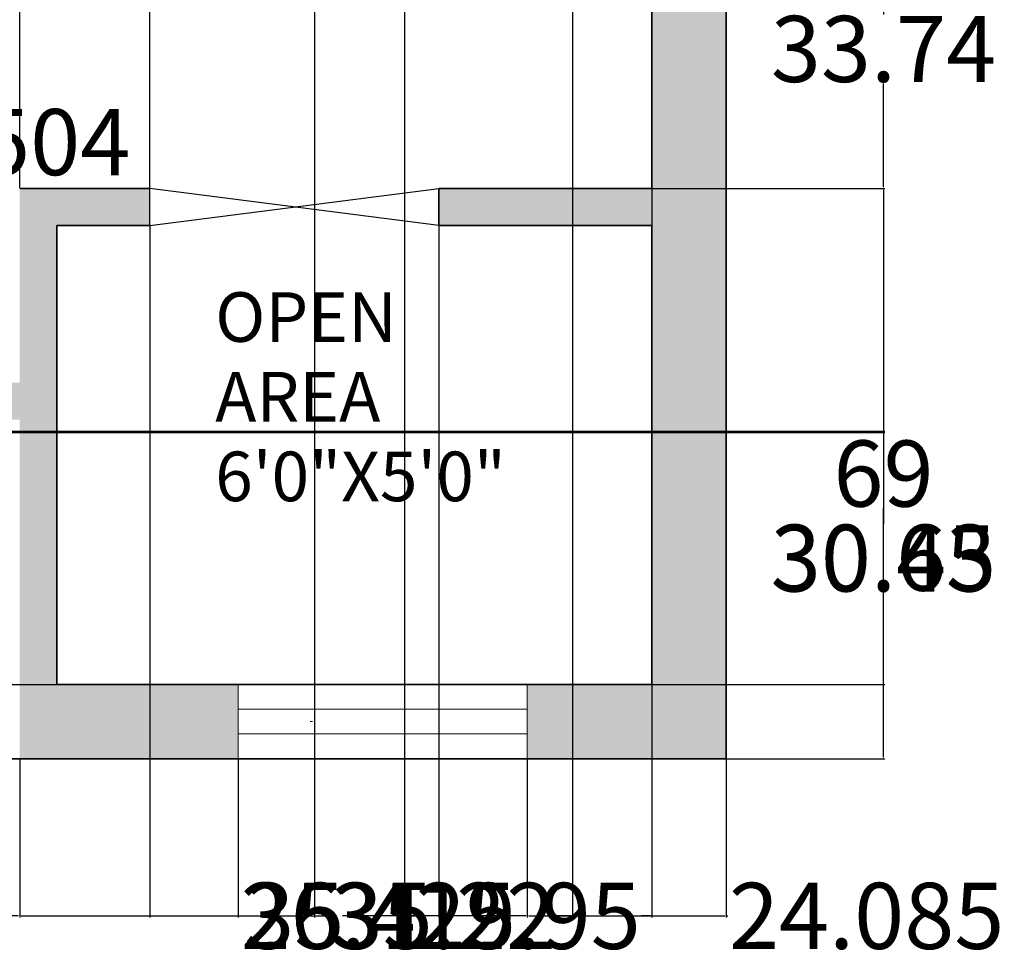
# Model space of a CAD drawing. Units: inches. Extents: x -24 to 368, y -370 to 58.
# Tile 4 of 9: x 237 to 356, y -369 to -255. Entities that reach past the tile are written whole.
import ezdxf

# ---------------------------------------------------------------- set-up
doc = ezdxf.new("R2010")
doc.units = ezdxf.units.IN
doc.header["$MEASUREMENT"] = 0
for name, color, linetype, lineweight in [('A-ANNO-DIMS', 2, 'Continuous', 18), ('A-AREA-IDEN', 7, 'Continuous', 18), ('A-WALL', 7, 'Continuous', 35)]:
    doc.layers.add(name, color=color, linetype=linetype, lineweight=lineweight)
for name, color, linetype, lineweight, true_color in [('A-DOOR', 40, 'Continuous', 25, 0xf8d731), ('A-GLAZ', 30, 'Continuous', 18, 0xf26722), ('A-WALL-PATT', 18, 'Continuous', 13, 0x000000)]:
    doc.layers.add(name, color=color, linetype=linetype, lineweight=lineweight, true_color=true_color)
doc.styles.get("Standard").update_dxf_attribs({"font": 'arial.ttf'})
doc.dimstyles.get("Standard").update_dxf_attribs({"dimtxt": 8, "dimasz": 0.18, "dimexe": 0.18, "dimexo": 0.0625, "dimgap": 0.09, "dimtad": 0, "dimtih": 1, "dimtoh": 1, "dimdec": 4, "dimzin": 0, "dimdsep": 46, "dimlunit": 3, "dimtxsty": 'Standard', "dimcen": 0.09, "dimclre": 5, "dimclrt": 6, "dimadec": 0, "dimazin": 0, "dimtfac": 1, "dimtdec": 4, "dimtofl": 0, "dimtmove": 0, "dimatfit": 3, "dimfxl": 1, "dimtolj": 1, "dimtzin": 0, "dimarcsym": 0})

# ---------------------------------------------------------------- blocks, each defined once
blk = doc.blocks.new('*D29')
at = {"layer": 'A-ANNO-DIMS', "color": 5, "lineweight": -2, "transparency": 16777216}
for p, q in [((131.66, -344.42), (131.66, -363.55)), ((236.66, -344.42), (236.66, -363.55))]:
    blk.add_line(p, q, dxfattribs=at)
at = {"layer": 'A-ANNO-DIMS', "color": 0, "lineweight": -2, "transparency": 16777216}
for p, q in [((131.84, -363.37), (175.58, -363.37)), ((236.48, -363.37), (192.74, -363.37))]:
    blk.add_line(p, q, dxfattribs=at)
at = {"layer": 'A-ANNO-DIMS', "color": 0, "transparency": 16777216}
for points in [[(131.84, -363.34), (131.84, -363.4), (131.66, -363.37)], [(236.48, -363.34), (236.48, -363.4), (236.66, -363.37)]]:
    blk.add_solid(points, dxfattribs=at)
at = {"layer": 'Defpoints', "color": 0, "transparency": 16777216}
for p in [(131.66, -344.36), (236.66, -344.36), (236.66, -363.37)]:
    blk.add_point(p, dxfattribs=at)
at = {"layer": 'A-ANNO-DIMS', "color": 6, "transparency": 16777216, "insert": (184.16, -363.37), "char_height": 8, "attachment_point": 5}
blk.add_mtext('\\A1;105', dxfattribs=at)
blk = doc.blocks.new('*D30')
at = {"layer": 'A-ANNO-DIMS', "color": 5, "lineweight": -2, "transparency": 16777216}
for p, q in [((236.66, -344.42), (236.66, -363.55)), ((263.08, -344.42), (263.08, -363.55))]:
    blk.add_line(p, q, dxfattribs=at)
at = {"layer": 'A-ANNO-DIMS', "color": 0, "lineweight": -2, "transparency": 16777216}
for p, q in [((236.84, -363.37), (262.9, -363.37)), ((263.08, -363.37), (263.26, -363.37))]:
    blk.add_line(p, q, dxfattribs=at)
at = {"layer": 'A-ANNO-DIMS', "color": 0, "transparency": 16777216}
for points in [[(236.84, -363.34), (236.84, -363.4), (236.66, -363.37)], [(262.9, -363.34), (262.9, -363.4), (263.08, -363.37)]]:
    blk.add_solid(points, dxfattribs=at)
at = {"layer": 'Defpoints', "color": 0, "transparency": 16777216}
for p in [(236.66, -344.36), (263.08, -344.36), (263.08, -363.37)]:
    blk.add_point(p, dxfattribs=at)
at = {"layer": 'A-ANNO-DIMS', "color": 6, "transparency": 16777216, "insert": (280.05, -363.37), "char_height": 8, "attachment_point": 5}
blk.add_mtext('\\A1;26.415', dxfattribs=at)
blk = doc.blocks.new('*D31')
at = {"layer": 'A-ANNO-DIMS', "color": 5, "lineweight": -2, "transparency": 16777216}
for p, q in [((263.08, -344.42), (263.08, -363.55)), ((298.08, -344.42), (298.08, -363.55))]:
    blk.add_line(p, q, dxfattribs=at)
at = {"layer": 'A-ANNO-DIMS', "color": 0, "lineweight": -2, "transparency": 16777216}
for p, q in [((263.26, -363.37), (274.73, -363.37)), ((297.9, -363.37), (286.42, -363.37))]:
    blk.add_line(p, q, dxfattribs=at)
at = {"layer": 'A-ANNO-DIMS', "color": 0, "transparency": 16777216}
for points in [[(263.26, -363.34), (263.26, -363.4), (263.08, -363.37)], [(297.9, -363.34), (297.9, -363.4), (298.08, -363.37)]]:
    blk.add_solid(points, dxfattribs=at)
at = {"layer": 'Defpoints', "color": 0, "transparency": 16777216}
for p in [(263.08, -344.36), (298.08, -344.36), (298.08, -363.37)]:
    blk.add_point(p, dxfattribs=at)
at = {"layer": 'A-ANNO-DIMS', "color": 6, "transparency": 16777216, "insert": (280.58, -363.37), "char_height": 8, "attachment_point": 5}
blk.add_mtext('\\A1;35', dxfattribs=at)
blk = doc.blocks.new('*D32')
at = {"layer": 'A-ANNO-DIMS', "color": 5, "lineweight": -2, "transparency": 16777216}
for p, q in [((298.08, -344.42), (298.08, -363.55)), ((322.16, -344.42), (322.16, -363.55))]:
    blk.add_line(p, q, dxfattribs=at)
at = {"layer": 'A-ANNO-DIMS', "color": 0, "lineweight": -2, "transparency": 16777216}
for p, q in [((298.26, -363.37), (321.98, -363.37)), ((322.16, -363.37), (322.34, -363.37))]:
    blk.add_line(p, q, dxfattribs=at)
at = {"layer": 'A-ANNO-DIMS', "color": 0, "transparency": 16777216}
for points in [[(298.26, -363.34), (298.26, -363.4), (298.08, -363.37)], [(321.98, -363.34), (321.98, -363.4), (322.16, -363.37)]]:
    blk.add_solid(points, dxfattribs=at)
at = {"layer": 'Defpoints', "color": 0, "transparency": 16777216}
for p in [(298.08, -344.36), (322.16, -344.36), (322.16, -363.37)]:
    blk.add_point(p, dxfattribs=at)
at = {"layer": 'A-ANNO-DIMS', "color": 6, "transparency": 16777216, "insert": (339.14, -363.37), "char_height": 8, "attachment_point": 5}
blk.add_mtext('\\A1;24.085', dxfattribs=at)
blk = doc.blocks.new('*D33')
at = {"layer": 'A-ANNO-DIMS', "color": 5, "lineweight": -2, "transparency": 16777216}
for p, q in [((313.22, -275.36), (341.36, -275.36)), ((322.22, -344.36), (341.36, -344.36))]:
    blk.add_line(p, q, dxfattribs=at)
at = {"layer": 'A-ANNO-DIMS', "color": 0, "lineweight": -2, "transparency": 16777216}
for p, q in [((341.18, -275.54), (341.18, -305.68)), ((341.18, -344.18), (341.18, -314.03))]:
    blk.add_line(p, q, dxfattribs=at)
at = {"layer": 'A-ANNO-DIMS', "color": 0, "transparency": 16777216}
for points in [[(341.15, -275.54), (341.21, -275.54), (341.18, -275.36)], [(341.15, -344.18), (341.21, -344.18), (341.18, -344.36)]]:
    blk.add_solid(points, dxfattribs=at)
at = {"layer": 'Defpoints', "color": 0, "transparency": 16777216}
for p in [(313.16, -275.36), (341.18, -275.36), (322.16, -344.36)]:
    blk.add_point(p, dxfattribs=at)
at = {"layer": 'A-ANNO-DIMS', "color": 6, "transparency": 16777216, "insert": (341.18, -309.86), "char_height": 8, "attachment_point": 5}
blk.add_mtext('\\A1;69', dxfattribs=at)
blk = doc.blocks.new('*D34')
at = {"layer": 'A-ANNO-DIMS', "color": 5, "lineweight": -2, "transparency": 16777216}
for p, q in [((322.22, -241.61), (341.36, -241.61)), ((313.22, -275.36), (341.36, -275.36))]:
    blk.add_line(p, q, dxfattribs=at)
at = {"layer": 'A-ANNO-DIMS', "color": 0, "lineweight": -2, "transparency": 16777216}
for p, q in [((341.18, -241.79), (341.18, -254.31)), ((341.18, -275.18), (341.18, -262.66))]:
    blk.add_line(p, q, dxfattribs=at)
at = {"layer": 'A-ANNO-DIMS', "color": 0, "transparency": 16777216}
for points in [[(341.15, -241.79), (341.21, -241.79), (341.18, -241.61)], [(341.15, -275.18), (341.21, -275.18), (341.18, -275.36)]]:
    blk.add_solid(points, dxfattribs=at)
at = {"layer": 'Defpoints', "color": 0, "transparency": 16777216}
for p in [(322.16, -241.61), (341.18, -241.61), (313.16, -275.36)]:
    blk.add_point(p, dxfattribs=at)
at = {"layer": 'A-ANNO-DIMS', "color": 6, "transparency": 16777216, "insert": (341.18, -258.49), "char_height": 8, "attachment_point": 5}
blk.add_mtext('\\A1;33.74', dxfattribs=at)
blk = doc.blocks.new('*D43')
at = {"layer": 'A-ANNO-DIMS', "color": 5, "lineweight": -2, "transparency": 16777216}
for p, q in [((283.21, 24.58), (283.21, -363.55)), ((313.16, 24.58), (313.16, -363.55))]:
    blk.add_line(p, q, dxfattribs=at)
at = {"layer": 'A-ANNO-DIMS', "color": 0, "lineweight": -2, "transparency": 16777216}
for p, q in [((283.39, -363.37), (284.5, -363.37)), ((312.98, -363.37), (311.87, -363.37))]:
    blk.add_line(p, q, dxfattribs=at)
at = {"layer": 'A-ANNO-DIMS', "color": 0, "transparency": 16777216}
for points in [[(283.39, -363.34), (283.39, -363.4), (283.21, -363.37)], [(312.98, -363.34), (312.98, -363.4), (313.16, -363.37)]]:
    blk.add_solid(points, dxfattribs=at)
at = {"layer": 'Defpoints', "color": 0, "transparency": 16777216}
for p in [(283.21, 24.64), (313.16, 24.64), (313.16, -363.37)]:
    blk.add_point(p, dxfattribs=at)
at = {"layer": 'A-ANNO-DIMS', "color": 6, "transparency": 16777216, "insert": (298.19, -363.37), "char_height": 8, "attachment_point": 5}
blk.add_mtext('\\A1;29.95', dxfattribs=at)
blk = doc.blocks.new('*D46')
at = {"layer": 'A-ANNO-DIMS', "color": 5, "lineweight": -2, "transparency": 16777216}
for p, q in [((13.22, -304.91), (341.36, -304.91)), ((13.22, -335.36), (341.36, -335.36))]:
    blk.add_line(p, q, dxfattribs=at)
at = {"layer": 'A-ANNO-DIMS', "color": 0, "lineweight": -2, "transparency": 16777216}
for p, q in [((341.18, -305.09), (341.18, -315.95)), ((341.18, -335.18), (341.18, -324.31))]:
    blk.add_line(p, q, dxfattribs=at)
at = {"layer": 'A-ANNO-DIMS', "color": 0, "transparency": 16777216}
for points in [[(341.15, -305.09), (341.21, -305.09), (341.18, -304.91)], [(341.15, -335.18), (341.21, -335.18), (341.18, -335.36)]]:
    blk.add_solid(points, dxfattribs=at)
at = {"layer": 'Defpoints', "color": 0, "transparency": 16777216}
for p in [(13.16, -304.91), (341.18, -304.91), (13.16, -335.36)]:
    blk.add_point(p, dxfattribs=at)
at = {"layer": 'A-ANNO-DIMS', "color": 6, "transparency": 16777216, "insert": (341.18, -320.13), "char_height": 8, "attachment_point": 5}
blk.add_mtext('\\A1;30.45', dxfattribs=at)
blk = doc.blocks.new('*D61')
at = {"layer": 'A-ANNO-DIMS', "color": 5, "lineweight": -2, "transparency": 16777216}
for p, q in [((236.66, -275.29), (236.66, 52.85)), ((252.39, -275.29), (252.39, 52.85))]:
    blk.add_line(p, q, dxfattribs=at)
at = {"layer": 'A-ANNO-DIMS', "color": 0, "lineweight": -2, "transparency": 16777216}
for p, q in [((236.84, 52.67), (252.21, 52.67)), ((252.39, 52.67), (252.57, 52.67))]:
    blk.add_line(p, q, dxfattribs=at)
at = {"layer": 'A-ANNO-DIMS', "color": 0, "transparency": 16777216}
for points in [[(236.84, 52.7), (236.84, 52.64), (236.66, 52.67)], [(252.21, 52.7), (252.21, 52.64), (252.39, 52.67)]]:
    blk.add_solid(points, dxfattribs=at)
at = {"layer": 'Defpoints', "color": 0, "transparency": 16777216}
for p in [(252.39, 52.67), (236.66, -275.36), (252.39, -275.36)]:
    blk.add_point(p, dxfattribs=at)
at = {"layer": 'A-ANNO-DIMS', "color": 6, "transparency": 16777216, "insert": (265.78, 52.67), "char_height": 8, "attachment_point": 5}
blk.add_mtext('\\A1;15.73', dxfattribs=at)
blk = doc.blocks.new('*D62')
at = {"layer": 'A-ANNO-DIMS', "color": 5, "lineweight": -2, "transparency": 16777216}
for p, q in [((252.39, -279.92), (252.39, -363.55)), ((287.39, -279.92), (287.39, -363.55))]:
    blk.add_line(p, q, dxfattribs=at)
at = {"layer": 'A-ANNO-DIMS', "color": 0, "lineweight": -2, "transparency": 16777216}
for p, q in [((252.57, -363.37), (264.04, -363.37)), ((287.21, -363.37), (275.74, -363.37))]:
    blk.add_line(p, q, dxfattribs=at)
at = {"layer": 'A-ANNO-DIMS', "color": 0, "transparency": 16777216}
for points in [[(252.57, -363.34), (252.57, -363.4), (252.39, -363.37)], [(287.21, -363.34), (287.21, -363.4), (287.39, -363.37)]]:
    blk.add_solid(points, dxfattribs=at)
at = {"layer": 'Defpoints', "color": 0, "transparency": 16777216}
for p in [(252.39, -279.86), (287.39, -279.86), (287.39, -363.37)]:
    blk.add_point(p, dxfattribs=at)
at = {"layer": 'A-ANNO-DIMS', "color": 6, "transparency": 16777216, "insert": (269.89, -363.37), "char_height": 8, "attachment_point": 5}
blk.add_mtext('\\A1;35', dxfattribs=at)
blk = doc.blocks.new('*D64')
at = {"layer": 'A-ANNO-DIMS', "color": 5, "lineweight": -2, "transparency": 16777216}
for p, q in [((105.73, -304.73), (341.36, -304.73)), ((106.02, -335.36), (341.36, -335.36))]:
    blk.add_line(p, q, dxfattribs=at)
at = {"layer": 'A-ANNO-DIMS', "color": 0, "lineweight": -2, "transparency": 16777216}
for p, q in [((341.18, -304.91), (341.18, -315.86)), ((341.18, -335.18), (341.18, -324.22))]:
    blk.add_line(p, q, dxfattribs=at)
at = {"layer": 'A-ANNO-DIMS', "color": 0, "transparency": 16777216}
for points in [[(341.15, -304.91), (341.21, -304.91), (341.18, -304.73)], [(341.15, -335.18), (341.21, -335.18), (341.18, -335.36)]]:
    blk.add_solid(points, dxfattribs=at)
at = {"layer": 'Defpoints', "color": 0, "transparency": 16777216}
for p in [(105.67, -304.73), (341.18, -304.73), (105.95, -335.36)]:
    blk.add_point(p, dxfattribs=at)
at = {"layer": 'A-ANNO-DIMS', "color": 6, "transparency": 16777216, "insert": (341.18, -320.04), "char_height": 8, "attachment_point": 5}
blk.add_mtext('\\A1;30.63', dxfattribs=at)
blk = doc.blocks.new('*D67')
at = {"layer": 'A-ANNO-DIMS', "color": 5, "lineweight": -2, "transparency": 16777216}
for p, q in [((303.55, -244.87), (303.55, -363.55)), ((272.33, -249.36), (272.33, -363.55))]:
    blk.add_line(p, q, dxfattribs=at)
at = {"layer": 'A-ANNO-DIMS', "color": 0, "lineweight": -2, "transparency": 16777216}
for p, q in [((272.51, -363.37), (274.4, -363.37)), ((303.37, -363.37), (301.49, -363.37))]:
    blk.add_line(p, q, dxfattribs=at)
at = {"layer": 'A-ANNO-DIMS', "color": 0, "transparency": 16777216}
for points in [[(272.51, -363.34), (272.51, -363.4), (272.33, -363.37)], [(303.37, -363.34), (303.37, -363.4), (303.55, -363.37)]]:
    blk.add_solid(points, dxfattribs=at)
at = {"layer": 'Defpoints', "color": 0, "transparency": 16777216}
for p in [(303.55, -244.81), (272.33, -249.3), (303.55, -363.37)]:
    blk.add_point(p, dxfattribs=at)
at = {"layer": 'A-ANNO-DIMS', "color": 6, "transparency": 16777216, "insert": (287.94, -363.37), "char_height": 8, "attachment_point": 5}
blk.add_mtext('\\A1;31.22', dxfattribs=at)
blk = doc.blocks.new('*D71')
at = {"layer": 'A-ANNO-DIMS', "color": 0, "lineweight": -2, "transparency": 16777216}
for p, q in [((209.23, -269.76), (196.73, -282.05)), ((209.41, -269.76), (209.23, -269.76))]:
    blk.add_line(p, q, dxfattribs=at)
at = {"layer": 'A-ANNO-DIMS', "color": 5, "lineweight": -2, "transparency": 16777216}
for p, q in [((175.48, -302.86), (175.66, -302.86)), ((175.57, -302.95), (175.57, -302.77))]:
    blk.add_line(p, q, dxfattribs=at)
at = {"layer": 'A-ANNO-DIMS', "color": 0, "transparency": 16777216}
blk.add_solid([(196.71, -282.03), (196.76, -282.07), (196.61, -282.17)], dxfattribs=at)
at = {"layer": 'Defpoints', "color": 0, "transparency": 16777216}
for p in [(196.61, -282.17), (175.57, -302.86)]:
    blk.add_point(p, dxfattribs=at)
at = {"layer": 'A-ANNO-DIMS', "color": 6, "transparency": 16777216, "insert": (229.92, -269.76), "char_height": 8, "attachment_point": 5}
blk.add_mtext('\\A1;R29.504', dxfattribs=at)

msp = doc.modelspace()

# ---------------------------------------------------------------- hatches: boundary and pattern name
at = {"layer": 'A-WALL-PATT'}
h = msp.add_hatch(color=256, dxfattribs=at)
h.dxf.hatch_style = 1
h.paths.add_polyline_path([(13.1621, -93.8573), (80.4499, -93.8573), (80.4499, -89.3573), (13.1621, -89.3573), (13.1621, -61.0987), (4.1621, -61.0987), (4.1621, -149.8573), (13.1621, -149.8573)])
h.paths.add_polyline_path([(146.5668, -27.3573), (133.1621, -27.3573), (133.1621, 10.3323), (133.1272, 10.3313), (133.1621, 24.6427), (139.8141, 24.6427), (139.8141, 33.6427), (95.3329, 33.6427), (95.3329, 24.6427), (128.6621, 24.6427), (128.6621, -89.3573), (127.4499, -89.3573), (127.4499, -93.8573), (133.1621, -93.8573), (133.1621, -31.8573), (146.5668, -31.8573)])
h.paths.add_polyline_path([(197.6621, 24.6427), (236.2134, 24.6427), (236.2134, 33.6427), (169.8141, 33.6427), (169.8141, 24.6427), (193.1621, 24.6427), (193.1621, -27.3573), (181.5668, -27.3573), (181.5668, -31.8573), (193.1621, -31.8573), (193.1621, -95.8573), (199.2127, -95.8573), (199.2127, -91.3573), (197.6621, -91.3573)])
h.paths.add_polyline_path([(322.1621, -52.531), (313.1621, -52.531), (313.1621, -91.3573), (246.2127, -91.3573), (246.2127, -95.8573), (246.6621, -95.8573), (246.6621, -104.9077), (251.1621, -104.9077), (251.1621, -95.8573), (313.1621, -95.8573), (313.1621, -105.6922), (317.6621, -105.6922), (322.1621, -105.6922)])
h.paths.add_polyline_path([(322.1621, -135.6922), (313.1621, -135.6922), (313.1621, -147.8573), (251.1621, -147.8573), (251.1621, -139.9077), (246.6621, -139.9077), (246.6621, -147.8573), (199.43, -147.8573), (199.43, -152.3573), (313.1621, -152.3573), (313.1621, -194.6142), (317.6621, -194.6142), (322.1621, -194.6142)])
h.paths.add_polyline_path([(322.1621, -241.6142), (313.1621, -241.6142), (313.1621, -275.3573), (287.3912, -275.3573), (287.3912, -279.8573), (313.1621, -279.8573), (313.1621, -335.3573), (298.077, -335.3573), (298.077, -344.3573), (322.1621, -344.3573)])
h.paths.add_polyline_path([(263.077, -335.3573), (241.1621, -335.3573), (241.1621, -279.8573), (252.3912, -279.8573), (252.3912, -275.3573), (236.6621, -275.3573), (236.6621, -298.8573), (234.5689, -298.8573), (234.5689, -303.3573), (236.6621, -303.3573), (236.6621, -344.3573), (263.077, -344.3573), (263.077, -339.8573)])
h.paths.add_polyline_path([(175.5689, -298.8573), (131.6621, -298.8573), (131.6621, -152.3573), (164.43, -152.3573), (164.43, -147.8573), (127.1621, -147.8573), (127.1621, -232.8573), (117.1621, -232.8573), (117.1621, -237.3573), (127.1621, -237.3573), (127.1621, -335.3573), (84.4055, -335.3573), (84.4055, -344.3573), (131.6621, -344.3573), (131.6621, -303.3573), (175.5689, -303.3573)])
h.paths.add_polyline_path([(70.1621, -232.8573), (13.1621, -232.8573), (13.1621, -196.8573), (4.1621, -196.8573), (4.1621, -257.9061), (13.1621, -257.9061), (13.1621, -237.3573), (70.1621, -237.3573)])
h.paths.add_polyline_path([(13.1621, -304.9061), (4.1621, -304.9061), (4.1621, -344.3573), (37.4055, -344.3573), (37.4055, -335.3573), (13.1621, -335.3573)])
h.paths.add_polyline_path([(322.1621, 33.6427), (283.2134, 33.6427), (283.2134, 24.6427), (313.1621, 24.6427), (313.1621, 11.9273), (313.4656, 11.629), (313.1621, 11.629), (313.1621, -5.531), (322.1621, -5.531)])
h.paths.add_polyline_path([(48.3329, 33.6427), (4.1621, 33.6427), (4.1621, -14.0987), (13.1621, -14.0987), (13.1621, 24.6427), (48.3329, 24.6427)])

# ---------------------------------------------------------------- linework, layer by layer
at = {"layer": 'A-DOOR'}
for p, q in [((252.3912, -279.8573), (252.3912, -275.3573)), ((252.3912, -279.8573), (287.3912, -275.3573)), ((287.3912, -279.8573), (252.3912, -275.3573)), ((287.3912, -279.8573), (287.3912, -275.3573)), ((287.3912, -275.3573), (287.3912, -279.8573))]:
    msp.add_line(p, q, dxfattribs=at)
at = {"layer": 'A-GLAZ'}
for p, q in [((298.077, -335.3573), (263.077, -335.3573)), ((263.077, -335.3573), (263.077, -344.3573)), ((298.077, -344.3573), (298.077, -335.3573)), ((263.077, -338.3573), (298.077, -338.3573)), ((263.077, -338.3573), (298.077, -338.3573)), ((263.077, -344.3573), (263.077, -339.8573)), ((263.077, -339.8573), (263.077, -339.8573)), ((263.077, -339.8573), (263.077, -339.8573)), ((271.827, -339.8573), (272.0916, -339.8573)), ((272.0916, -339.8573), (272.0916, -339.8573)), ((272.0916, -339.8573), (272.0916, -339.8573)), ((263.077, -341.3573), (298.077, -341.3573)), ((263.077, -344.3573), (298.077, -344.3573))]:
    msp.add_line(p, q, dxfattribs=at)
at = {"layer": 'A-WALL'}
for p, q in [((322.1621, 33.6427), (322.1621, -344.3573)), ((313.1621, -232.8573), (313.1621, -275.3573)), ((252.3912, -275.3573), (236.6621, -275.3573)), ((313.1621, -275.3573), (287.3912, -275.3573)), ((241.1621, -279.8573), (241.1621, -335.3573)), ((252.3912, -279.8573), (241.1621, -279.8573)), ((313.1621, -279.8573), (287.3912, -279.8573)), ((313.1621, -279.8573), (313.1621, -335.3573)), ((313.1621, -335.3573), (241.1621, -335.3573)), ((322.1621, -344.3573), (4.1621, -344.3573))]:
    msp.add_line(p, q, dxfattribs=at)

# ---------------------------------------------------------------- texts
at = {"layer": 'A-AREA-IDEN'}
for s, p in [('OPEN', (260.3195, -293.9263)), ('AREA', (260.3195, -303.5648)), ('6\'0"X5\'0"', (260.3195, -313.2032))]:
    msp.add_text(s, height=6, dxfattribs=at).set_placement(p)

# ---------------------------------------------------------------- dimensions: what is measured, and where the dimension line sits
at = {"layer": 'A-ANNO-DIMS'}
for base, p1, p2, override, picture, middle in [((252.3912, 52.6658), (236.6621, -275.3573), (252.3912, -275.3573), {"dimdec": 2, "dimlfac": 1, "dimrnd": 0, "dimzin": 0, "dimdsep": 46, "dimlunit": 2}, '*D61', (265.7827, 52.6658)), ((313.1621, -363.3723), (283.2134, 24.6427), (313.1621, 24.6427), {"dimdec": 2, "dimlfac": 1, "dimrnd": 0, "dimzin": 0, "dimdsep": 46, "dimlunit": 2}, '*D43', (298.1877, -363.3723)), ((303.5496, -363.3723), (272.3319, -249.2987), (303.5496, -244.8091), {"dimdec": 2, "dimlfac": 1, "dimrnd": 0, "dimzin": 0, "dimdsep": 46, "dimlunit": 2}, '*D67', (287.9407, -363.3723)), ((287.3912, -363.3723), (252.3912, -279.8573), (287.3912, -279.8573), {"dimdec": 0, "dimlfac": 1, "dimrnd": 0, "dimzin": 0, "dimdsep": 46, "dimlunit": 2}, '*D62', (269.8912, -363.3723)), ((236.6621, -363.3723), (131.6621, -344.3573), (236.6621, -344.3573), {"dimdec": 0, "dimlfac": 1, "dimrnd": 0, "dimzin": 0, "dimdsep": 46, "dimlunit": 2}, '*D29', (184.1621, -363.3723)), ((263.077, -363.3723), (236.6621, -344.3573), (263.077, -344.3573), {"dimdec": 3, "dimlfac": 1, "dimrnd": 0, "dimzin": 0, "dimdsep": 46, "dimlunit": 2}, '*D30', (280.0509, -363.3723)), ((298.077, -363.3723), (263.077, -344.3573), (298.077, -344.3573), {"dimdec": 0, "dimlfac": 1, "dimrnd": 0, "dimzin": 0, "dimdsep": 46, "dimlunit": 2}, '*D31', (280.577, -363.3723)), ((322.1621, -363.3723), (298.077, -344.3573), (322.1621, -344.3573), {"dimdec": 3, "dimlfac": 1, "dimrnd": 0, "dimzin": 0, "dimdsep": 46, "dimlunit": 2}, '*D32', (339.1361, -363.3723))]:
    dim = msp.add_linear_dim(base=base, p1=p1, p2=p2, dimstyle='Standard', override=override, dxfattribs=at)
    dim.commit()
    dim.dimension.update_dxf_attribs({"geometry": picture, "text_midpoint": middle})
for base, p1, p2, override, picture, middle in [((341.1771, -241.6142), (313.1621, -275.3573), (322.1621, -241.6142), {"dimdec": 2, "dimlfac": 1, "dimrnd": 0, "dimzin": 0, "dimdsep": 46, "dimlunit": 2}, '*D34', (341.1771, -258.4858)), ((341.1771, -275.3573), (322.1621, -344.3573), (313.1621, -275.3573), {"dimdec": 0, "dimlfac": 1, "dimrnd": 0, "dimzin": 0, "dimdsep": 46, "dimlunit": 2}, '*D33', (341.1771, -309.8573)), ((341.1771, -304.9061), (13.1621, -335.3573), (13.1621, -304.9061), {"dimdec": 2, "dimlfac": 1, "dimrnd": 0, "dimzin": 0, "dimdsep": 46, "dimlunit": 2}, '*D46', (341.1771, -320.1317)), ((341.1771, -304.7252), (105.953, -335.3573), (105.6669, -304.7252), {"dimdec": 2, "dimlfac": 1, "dimrnd": 0, "dimzin": 0, "dimdsep": 46, "dimlunit": 2}, '*D64', (341.1771, -320.0412))]:
    dim = msp.add_linear_dim(base=base, p1=p1, p2=p2, angle=90, dimstyle='Standard', override=override, dxfattribs=at)
    dim.commit()
    dim.dimension.update_dxf_attribs({"geometry": picture, "text_midpoint": middle})
dim = msp.add_radius_dim(center=(175.5689, -302.8615), mpoint=(196.606, -282.175), dimstyle='Standard', override={"dimdec": 3, "dimlfac": 1, "dimrnd": 0, "dimzin": 0, "dimdsep": 46, "dimlunit": 2}, dxfattribs=at)
dim.commit()
dim.dimension.update_dxf_attribs({"geometry": '*D71', "text_midpoint": (229.9158, -269.763), "dimtype": 164})

doc.saveas('drawing.dxf')
